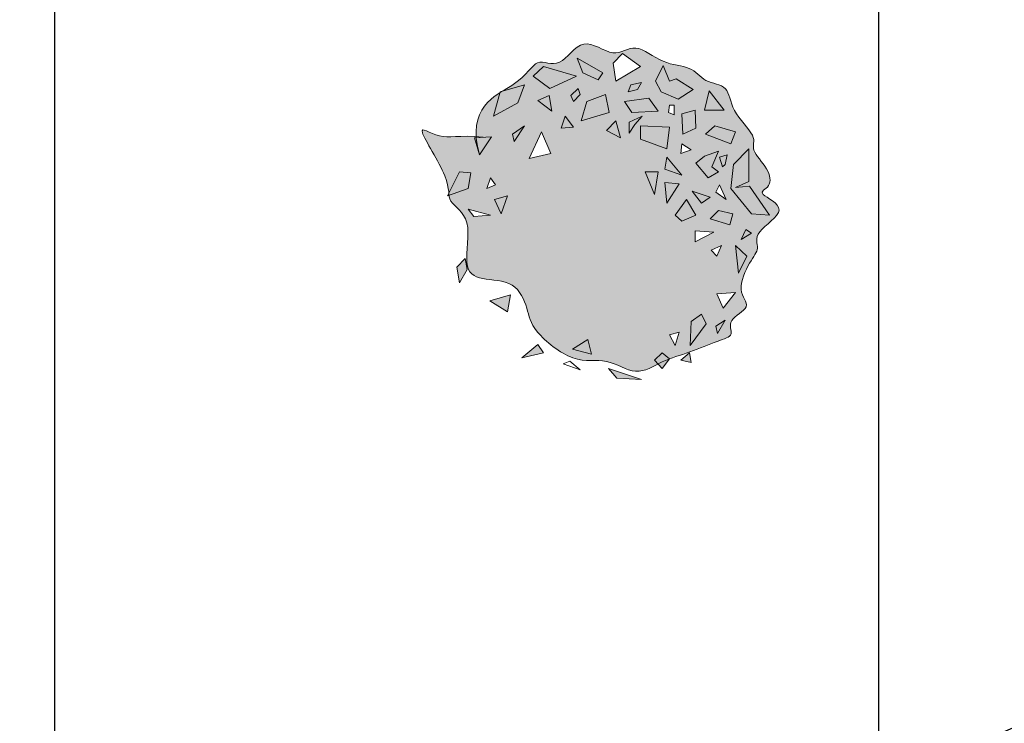
# Model space of a CAD drawing. Units: metres. Extents: x 4298.5 to 4325.2, y 2075 to 2095.8.
# Tile 4 of 35: x 4305.827 to 4307.62, y 2077.753 to 2079.034. Entities that reach past the tile are written whole.
import ezdxf

# ---------------------------------------------------------------- set-up
doc = ezdxf.new("R2010")
doc.units = ezdxf.units.M
doc.layers.add('A-ANNO-DIMS', color=2, linetype='Continuous', lineweight=18)
doc.layers.add('L-PLNT', color=94, linetype='Continuous', lineweight=13)
doc.layers.add('L-PLNT-PATT', color=116, linetype='Continuous', lineweight=13, true_color=0x13823e)
doc.styles.get("Standard").update_dxf_attribs({"font": 'arial.ttf'})
doc.dimstyles.get("Standard").update_dxf_attribs({"dimtxt": 0.18, "dimasz": 0.18, "dimexe": 0.18, "dimexo": 0.0625, "dimgap": 0.09, "dimtad": 0, "dimtih": 1, "dimtoh": 1, "dimdec": 4, "dimzin": 0, "dimdsep": 46, "dimtxsty": 'Standard', "dimcen": 0.09, "dimadec": 0, "dimazin": 0, "dimtfac": 1, "dimtdec": 4, "dimtofl": 0, "dimtmove": 0, "dimatfit": 3, "dimfxl": 1, "dimtolj": 1, "dimtzin": 0, "dimarcsym": 0})

# ---------------------------------------------------------------- blocks, each defined once
blk = doc.blocks.new('*U9')
for points in [[(1.237, 12.003), (0.562, 11.31), (0.764, 10.013), (2.519, 11.051)], [(-2.003, 11.656), (-1.598, 10.618), (-0.518, 10.099), (-0.181, 10.618), (-0.788, 10.964)], [(-4.432, 11.051), (-5.175, 10.359), (-3.96, 9.493), (-2.07, 10.359)], [(4.139, 11.137), (3.599, 10.013), (4.004, 9.234), (5.218, 8.715), (6.298, 9.407), (5.083, 10.186), (4.611, 10.013)], [(2.586, 9.926), (1.844, 9.753), (1.642, 9.234), (2.316, 9.407)], [(-5.782, 9.753), (-7.537, 9.234), (-8.009, 7.504), (-6.255, 8.455)], [(-1.935, 9.493), (-2.475, 8.974), (-2.273, 8.542), (-1.8, 9.061)], [(7.446, 9.32), (7.108, 7.936), (8.525, 7.936)], [(-4.837, 8.628), (-3.825, 7.85), (-4.027, 8.974)], [(0.022, 9.061), (-1.328, 8.542), (-1.733, 7.157), (0.292, 7.763)], [(1.372, 8.542), (3.126, 8.801), (3.801, 7.85), (1.912, 7.763)], [(4.611, 8.282), (4.544, 7.763), (4.949, 7.59), (4.949, 8.282)], [(6.433, 7.936), (5.488, 7.676), (5.556, 6.206), (6.501, 6.638)], [(-2.88, 7.504), (-3.15, 6.638), (-2.273, 6.725)], [(0.764, 7.157), (0.089, 6.465), (1.102, 5.946)], [(1.709, 6.292), (1.709, 7.071), (2.654, 7.504), (2.114, 6.898)], [(-5.782, 6.811), (-6.659, 6.206), (-6.524, 5.687)], [(-4.567, 6.379), (-5.445, 4.475), (-3.892, 4.821)], [(2.519, 6.811), (2.519, 5.86), (4.409, 5.167), (4.611, 6.725)], [(7.851, 6.811), (7.176, 6.206), (8.998, 5.514), (9.335, 6.379)], [(-8.144, 6.033), (-9.359, 5.946), (-9.022, 4.735)], [(5.488, 5.514), (5.421, 4.821), (6.163, 5.081)], [(8.12, 4.994), (7.108, 4.648), (6.501, 4.129), (7.378, 3.091), (8.12, 3.524), (7.648, 3.87)], [(10.28, 5.167), (9.2, 4.043), (8.998, 2.312), (10.482, 0.495), (11.765, 0.409), (10.348, 2.485), (9.335, 2.399), (10.28, 2.831)], [(4.409, 4.562), (4.274, 3.697), (5.488, 3.264)], [(8.728, 4.735), (8.188, 4.562), (8.39, 3.87), (8.593, 4.043)], [(-11.316, 1.793), (-9.831, 2.312), (-9.629, 3.437), (-10.439, 3.524)], [(-8.212, 3.091), (-8.482, 2.312), (-7.874, 2.572)], [(3.531, 1.88), (2.856, 3.524), (3.801, 3.524)], [(4.274, 2.745), (5.286, 2.658), (4.409, 1.274)], [(7.513, 1.707), (6.906, 1.274), (6.231, 2.139)], [(8.188, 2.572), (7.918, 2.053), (8.66, 1.534)], [(-6.997, 1.793), (-7.942, 1.534), (-7.469, 0.495)], [(5.826, 1.534), (5.016, 0.409), (5.488, -0.024), (6.501, 0.409)], [(-8.212, 0.409), (-9.426, 0.322), (-9.831, 0.841)], [(8.12, 0.755), (7.513, 0.149), (8.93, -0.283), (9.133, 0.495)], [(10.078, -0.629), (9.74, -1.322), (10.482, -0.889)], [(7.783, -0.803), (6.433, -1.495), (6.433, -0.716)], [(8.323, -1.754), (7.985, -2.533), (7.581, -2.1)], [(9.335, -1.754), (9.538, -3.744), (10.145, -2.533)], [(-10.034, -2.706), (-10.641, -3.312), (-10.439, -4.436), (-9.899, -3.485)], [(-8.279, -5.734), (-6.794, -5.302), (-6.997, -6.513)], [(9.335, -5.129), (8.458, -6.253), (7.985, -5.215)], [(6.096, -8.935), (6.163, -7.205), (6.906, -6.686), (7.243, -7.378)], [(8.053, -8.07), (8.593, -7.118), (7.918, -7.551)], [(5.286, -7.984), (4.611, -8.157), (5.016, -8.935)], [(-4.837, -8.849), (-4.432, -9.454), (-5.985, -9.801)], [(-2.34, -9.195), (-1.26, -8.503), (-0.99, -9.541)], [(4.071, -9.454), (3.531, -9.974), (4.071, -10.579), (4.611, -9.887)], [(6.028, -9.454), (5.421, -9.974), (6.163, -10.147)], [(-2.543, -10.06), (-3.015, -10.233), (-1.8, -10.666)], [(0.224, -10.579), (0.832, -11.272), (2.586, -11.358)]]:
    blk.add_lwpolyline(points, close=True)
blk = doc.blocks.new('*D47')
at = {"layer": 'A-ANNO-DIMS', "color": 0, "lineweight": -2, "transparency": 16777216}
for p, q in [((4300.4306, 2084.4956), (4300.4306, 2074.9896)), ((4322.8106, 2084.4956), (4322.8106, 2074.9896)), ((4300.6106, 2075.1696), (4311.2252, 2075.1696)), ((4322.6306, 2075.1696), (4312.016, 2075.1696))]:
    blk.add_line(p, q, dxfattribs=at)
at = {"layer": 'A-ANNO-DIMS', "color": 0, "transparency": 16777216}
for points in [[(4300.6106, 2075.1996), (4300.6106, 2075.1396), (4300.4306, 2075.1696)], [(4322.6306, 2075.1996), (4322.6306, 2075.1396), (4322.8106, 2075.1696)]]:
    blk.add_solid(points, dxfattribs=at)
at = {"layer": 'Defpoints', "color": 0, "transparency": 16777216}
for p in [(4300.4306, 2084.5581), (4322.8106, 2084.5581), (4322.8106, 2075.1696)]:
    blk.add_point(p, dxfattribs=at)
at = {"layer": 'A-ANNO-DIMS', "color": 0, "transparency": 16777216, "insert": (4311.6206, 2075.1696), "char_height": 0.18, "attachment_point": 5}
blk.add_mtext('\\A1;22.38', dxfattribs=at)
blk = doc.blocks.new('*D54')
at = {"layer": 'A-ANNO-DIMS', "color": 0, "lineweight": -2, "transparency": 16777216}
for p, q in [((4305.5981, 2079.8281), (4299.0921, 2079.8281)), ((4299.2721, 2079.6481), (4299.2721, 2078.26)), ((4299.2721, 2076.5081), (4299.2721, 2077.8961)), ((4309.0981, 2076.3281), (4299.0921, 2076.3281))]:
    blk.add_line(p, q, dxfattribs=at)
at = {"layer": 'A-ANNO-DIMS', "color": 0, "transparency": 16777216}
for points in [[(4299.2421, 2079.6481), (4299.3021, 2079.6481), (4299.2721, 2079.8281)], [(4299.2421, 2076.5081), (4299.3021, 2076.5081), (4299.2721, 2076.3281)]]:
    blk.add_solid(points, dxfattribs=at)
at = {"layer": 'Defpoints', "color": 0, "transparency": 16777216}
for p in [(4305.6606, 2079.8281), (4299.2721, 2076.3281), (4309.1606, 2076.3281)]:
    blk.add_point(p, dxfattribs=at)
at = {"layer": 'A-ANNO-DIMS', "color": 0, "transparency": 16777216, "insert": (4299.2721, 2078.0781), "char_height": 0.18, "attachment_point": 5}
blk.add_mtext('\\A1;3.5', dxfattribs=at)
blk = doc.blocks.new('*D59')
at = {"layer": 'A-ANNO-DIMS', "color": 0, "lineweight": -2, "transparency": 16777216}
for p, q in [((4305.8906, 2079.9956), (4305.8906, 2074.9896)), ((4307.3906, 2079.9956), (4307.3906, 2074.9896)), ((4306.0706, 2075.1696), (4306.3945, 2075.1696)), ((4307.2106, 2075.1696), (4306.8866, 2075.1696))]:
    blk.add_line(p, q, dxfattribs=at)
at = {"layer": 'A-ANNO-DIMS', "color": 0, "transparency": 16777216}
for points in [[(4306.0706, 2075.1996), (4306.0706, 2075.1396), (4305.8906, 2075.1696)], [(4307.2106, 2075.1996), (4307.2106, 2075.1396), (4307.3906, 2075.1696)]]:
    blk.add_solid(points, dxfattribs=at)
at = {"layer": 'Defpoints', "color": 0, "transparency": 16777216}
for p in [(4305.8906, 2080.0581), (4307.3906, 2080.0581), (4307.3906, 2075.1696)]:
    blk.add_point(p, dxfattribs=at)
at = {"layer": 'A-ANNO-DIMS', "color": 0, "transparency": 16777216, "insert": (4306.6406, 2075.1696), "char_height": 0.18, "attachment_point": 5}
blk.add_mtext('\\A1;1.5', dxfattribs=at)
blk = doc.blocks.new('*D78')
at = {"layer": 'A-ANNO-DIMS', "color": 0, "lineweight": -2, "transparency": 16777216}
for p, q in [((4312.4969, 2079.7393), (4312.4969, 2079.9193)), ((4312.4069, 2079.8293), (4312.5869, 2079.8293)), ((4305.3847, 2076.7806), (4307.8863, 2077.853)), ((4305.2047, 2076.7806), (4305.3847, 2076.7806))]:
    blk.add_line(p, q, dxfattribs=at)
at = {"layer": 'A-ANNO-DIMS', "color": 0, "transparency": 16777216}
blk.add_solid([(4307.8745, 2077.8806), (4307.8981, 2077.8254), (4308.0518, 2077.9239)], dxfattribs=at)
at = {"layer": 'Defpoints', "color": 0, "transparency": 16777216}
for p in [(4312.4969, 2079.8293), (4308.0518, 2077.9239)]:
    blk.add_point(p, dxfattribs=at)
at = {"layer": 'A-ANNO-DIMS', "color": 0, "transparency": 16777216, "insert": (4304.53, 2076.7806), "char_height": 0.18, "attachment_point": 5}
blk.add_mtext('\\A1;2X R4.836', dxfattribs=at)

msp = doc.modelspace()

# ---------------------------------------------------------------- hatches: boundary and pattern name
at = {"layer": 'L-PLNT-PATT'}
h = msp.add_hatch(color=256, dxfattribs=at)
h.dxf.hatch_style = 1
edge = h.paths.add_edge_path()
edge.add_spline(control_points=[(4306.9894, 2078.4071), (4306.992, 2078.4084), (4307.0106, 2078.4177), (4307.0464, 2078.4275), (4307.1009, 2078.4508), (4307.1303, 2078.4584), (4307.1115, 2078.4868), (4307.1641, 2078.511), (4307.1304, 2078.5374), (4307.1574, 2078.5971), (4307.1761, 2078.6166), (4307.1595, 2078.6451), (4307.2337, 2078.6899), (4307.1638, 2078.7195), (4307.1965, 2078.7271), (4307.1925, 2078.7623), (4307.1544, 2078.7989), (4307.173, 2078.8182), (4307.1199, 2078.8692), (4307.1199, 2078.9153), (4307.0721, 2078.9186), (4307.0516, 2078.9505), (4306.9984, 2078.9505), (4306.9461, 2078.9959), (4306.9113, 2078.9588), (4306.8506, 2079.0096), (4306.8107, 2078.9395), (4306.7661, 2078.9695), (4306.7518, 2078.9301), (4306.7115, 2078.9071), (4306.7051, 2078.9032)], knot_values=[0.818571, 0.818571, 0.818571, 0.818571, 0.97924, 1.97924, 2.97924, 3.97924, 4.97924, 5.97924, 6.97924, 7.97924, 8.97924, 9.97924, 10.97924, 11.97924, 12.97924, 13.97924, 14.97924, 15.97924, 16.97924, 17.97924, 18.97924, 19.97924, 20.97924, 21.97924, 22.97924, 23.97924, 24.97924, 25.97924, 26.97924, 27.16067, 27.16067, 27.16067, 27.16067], degree=3, periodic=0)
edge.add_line((4306.7051, 2078.9032), (4306.7464, 2078.9154))
edge.add_line((4306.7464, 2078.9154), (4306.7344, 2078.8824))
edge.add_line((4306.7344, 2078.8824), (4306.6898, 2078.8582))
edge.add_line((4306.6898, 2078.8582), (4306.7015, 2078.9008))
edge.add_spline(control_points=[(4306.7015, 2078.9008), (4306.6788, 2078.8862), (4306.6555, 2078.8652), (4306.6583, 2078.8208)], knot_values=[0.141368, 0.141368, 0.141368, 0.141368, 0.783694, 0.783694, 0.783694, 0.783694], degree=3, periodic=0)
edge.add_spline(control_points=[(4306.6583, 2078.8208), (4306.6622, 2078.8206), (4306.6665, 2078.8202), (4306.671, 2078.8198)], knot_values=[40.901028, 40.901028, 40.901028, 40.901028, 41, 41, 41, 41], degree=3, periodic=0)
edge.add_line((4306.671, 2078.8198), (4306.6864, 2078.8209))
edge.add_line((4306.6864, 2078.8209), (4306.6641, 2078.7879))
edge.add_line((4306.6641, 2078.7879), (4306.6556, 2078.8187))
edge.add_line((4306.6556, 2078.8187), (4306.6584, 2078.8189))
edge.add_spline(control_points=[(4306.6584, 2078.8189), (4306.6583, 2078.8195), (4306.6583, 2078.8202), (4306.6583, 2078.8208)], knot_values=[0.13204, 0.13204, 0.13204, 0.13204, 0.141368, 0.141368, 0.141368, 0.141368], degree=3, periodic=0)
edge.add_spline(control_points=[(4306.6583, 2078.8208), (4306.622, 2078.8232), (4306.5904, 2078.8133), (4306.5384, 2078.8553), (4306.6055, 2078.7528), (4306.6078, 2078.7259), (4306.6085, 2078.7184)], knot_values=[37.439141, 37.439141, 37.439141, 37.439141, 38.340169, 39.340169, 40.340169, 40.901028, 40.901028, 40.901028, 40.901028], degree=3, periodic=0)
edge.add_line((4306.6085, 2078.7184), (4306.6281, 2078.7572))
edge.add_line((4306.6281, 2078.7572), (4306.6487, 2078.7549))
edge.add_line((4306.6487, 2078.7549), (4306.6436, 2078.7264))
edge.add_line((4306.6436, 2078.7264), (4306.6089, 2078.7143))
edge.add_spline(control_points=[(4306.6089, 2078.7143), (4306.6094, 2078.7103), (4306.6125, 2078.6968), (4306.6539, 2078.6758), (4306.6324, 2078.5785), (4306.6646, 2078.5597), (4306.7309, 2078.5597), (4306.7536, 2078.5059), (4306.7571, 2078.4705), (4306.8381, 2078.4044), (4306.8964, 2078.4212), (4306.9468, 2078.3843), (4306.9759, 2078.4003), (4306.9894, 2078.4071)], knot_values=[27.16067, 27.16067, 27.16067, 27.16067, 27.490087, 28.490087, 29.490087, 30.490087, 31.490087, 32.490087, 33.490087, 34.490087, 35.490087, 36.490087, 37.329418, 37.329418, 37.329418, 37.329418], degree=3, periodic=0)
edge.add_line((4306.9894, 2078.4071), (4306.983, 2078.4143))
edge.add_line((4306.983, 2078.4143), (4306.9967, 2078.4275))
edge.add_line((4306.9967, 2078.4275), (4307.0104, 2078.4165))
h.paths.add_polyline_path([(4306.9658, 2078.7572), (4306.9898, 2078.7572), (4306.983, 2078.7154)], flags=16)
h.paths.add_polyline_path([(4307.0018, 2078.7374), (4307.0275, 2078.7352), (4307.0053, 2078.7)], flags=16)
h.paths.add_polyline_path([(4306.7944, 2078.7901), (4306.755, 2078.7813), (4306.7773, 2078.8297)], flags=16)
h.paths.add_polyline_path([(4306.9213, 2078.8187), (4306.8955, 2078.8319), (4306.9127, 2078.8494)], flags=16)
h.paths.add_polyline_path([(4307.0018, 2078.7615), (4307.0053, 2078.7835), (4307.0327, 2078.7505)], flags=16)
h.paths.add_polyline_path([(4307.0207, 2078.678), (4307.0413, 2078.7066), (4307.0584, 2078.678), (4307.0327, 2078.667)], flags=16)
h.paths.add_polyline_path([(4306.9573, 2078.8165), (4306.9573, 2078.8406), (4307.0104, 2078.8385), (4307.0053, 2078.7989)], flags=16)
h.paths.add_polyline_path([(4306.9367, 2078.8275), (4306.9367, 2078.8472), (4306.9607, 2078.8582), (4306.947, 2078.8428)], flags=16)
h.paths.add_polyline_path([(4306.8355, 2078.8385), (4306.8133, 2078.8362), (4306.8201, 2078.8582)], flags=16)
h.paths.add_polyline_path([(4306.8493, 2078.8494), (4306.8595, 2078.8846), (4306.8938, 2078.8978), (4306.9007, 2078.8648)], flags=16)
h.paths.add_polyline_path([(4306.7156, 2078.7132), (4306.7036, 2078.6802), (4306.6915, 2078.7066)], flags=16)
h.paths.add_polyline_path([(4307.0515, 2078.722), (4307.0841, 2078.711), (4307.0687, 2078.7)], flags=16)
h.paths.add_polyline_path([(4307.031, 2078.7901), (4307.0327, 2078.8077), (4307.0498, 2078.7967)], flags=16)
h.paths.add_polyline_path([(4306.9418, 2078.8648), (4306.9281, 2078.8846), (4306.9727, 2078.8912), (4306.9898, 2078.867)], flags=16)
h.paths.add_polyline_path([(4307.0567, 2078.6495), (4307.091, 2078.6472), (4307.0567, 2078.6297)], flags=16)
h.paths.add_polyline_path([(4306.6933, 2078.733), (4306.6778, 2078.7264), (4306.6847, 2078.7462)], flags=16)
h.paths.add_polyline_path([(4306.7961, 2078.867), (4306.7704, 2078.8868), (4306.791, 2078.8956)], flags=16)
h.paths.add_polyline_path([(4306.7276, 2078.8121), (4306.7241, 2078.8253), (4306.7464, 2078.8406)], flags=16)
h.paths.add_polyline_path([(4306.8355, 2078.8846), (4306.8304, 2078.8956), (4306.8441, 2078.9088), (4306.8476, 2078.8978)], flags=16)
h.paths.add_polyline_path([(4307.0584, 2078.7725), (4307.0738, 2078.7857), (4307.0995, 2078.7945), (4307.0875, 2078.7659), (4307.0995, 2078.7572), (4307.0807, 2078.7462)], flags=16)
h.paths.add_polyline_path([(4306.6847, 2078.678), (4306.6539, 2078.6758), (4306.6436, 2078.689)], flags=16)
h.paths.add_polyline_path([(4307.0344, 2078.8253), (4307.0327, 2078.8626), (4307.0567, 2078.8692), (4307.0584, 2078.8362)], flags=16)
h.paths.add_polyline_path([(4307.0841, 2078.6714), (4307.0995, 2078.6868), (4307.1253, 2078.6802), (4307.1201, 2078.6605)], flags=16)
h.paths.add_polyline_path([(4307.0087, 2078.8648), (4307.0104, 2078.878), (4307.019, 2078.878), (4307.019, 2078.8604)], flags=16)
h.paths.add_polyline_path([(4306.935, 2078.9022), (4306.9401, 2078.9154), (4306.959, 2078.9198), (4306.9521, 2078.9066)], flags=16)
h.paths.add_polyline_path([(4307.0944, 2078.7198), (4307.1012, 2078.733), (4307.1132, 2078.7066)], flags=16)
h.paths.add_polyline_path([(4307.0858, 2078.6143), (4307.1047, 2078.6231), (4307.0961, 2078.6033)], flags=16)
h.paths.add_polyline_path([(4306.8801, 2078.9242), (4306.8527, 2078.9373), (4306.8424, 2078.9637), (4306.8733, 2078.9461), (4306.8887, 2078.9373)], flags=16)
h.paths.add_polyline_path([(4306.9127, 2078.922), (4306.9075, 2078.9549), (4306.9247, 2078.9725), (4306.9573, 2078.9483)], flags=16)
h.paths.add_polyline_path([(4306.7927, 2078.9088), (4306.7618, 2078.9308), (4306.7807, 2078.9483), (4306.8407, 2078.9308)], flags=16)
h.paths.add_polyline_path([(4307.0755, 2078.8253), (4307.0927, 2078.8406), (4307.1304, 2078.8297), (4307.1218, 2078.8077)], flags=16)
h.paths.add_polyline_path([(4306.995, 2078.9022), (4306.9847, 2078.922), (4306.9984, 2078.9505), (4307.0104, 2078.922), (4307.0224, 2078.9264), (4307.0532, 2078.9066), (4307.0258, 2078.889)], flags=16)
h.paths.add_polyline_path([(4307.1064, 2078.7659), (4307.1012, 2078.7835), (4307.115, 2078.7879), (4307.1115, 2078.7703)], flags=16)
h.paths.add_polyline_path([(4307.1218, 2078.7264), (4307.127, 2078.7703), (4307.1544, 2078.7989), (4307.1544, 2078.7395), (4307.1304, 2078.7286), (4307.1561, 2078.7308), (4307.1921, 2078.678), (4307.1595, 2078.6802)], flags=16)
h.paths.add_polyline_path([(4306.8613, 2078.4517), (4306.8681, 2078.4253), (4306.8338, 2078.4341)], flags=16)
h.paths.add_polyline_path([(4307.0738, 2078.8692), (4307.0824, 2078.9044), (4307.1098, 2078.8692)], flags=16)
h.paths.add_polyline_path([(4307.1304, 2078.6231), (4307.151, 2078.6033), (4307.1355, 2078.5725)], flags=16)
h.paths.add_polyline_path([(4307.1407, 2078.6341), (4307.1493, 2078.6517), (4307.1595, 2078.6451)], flags=16)
h.paths.add_polyline_path([(4307.0104, 2078.4605), (4307.0275, 2078.4648), (4307.0207, 2078.4407)], flags=16)
h.paths.add_polyline_path([(4307.0961, 2078.5352), (4307.1304, 2078.5374), (4307.1081, 2078.5088)], flags=16)
h.paths.add_polyline_path([(4307.0498, 2078.4846), (4307.0687, 2078.4978), (4307.0772, 2078.4802), (4307.0481, 2078.4407)], flags=16)
h.paths.add_polyline_path([(4307.0944, 2078.4758), (4307.1115, 2078.4868), (4307.0978, 2078.4627)], flags=16)
h = msp.add_hatch(color=256, dxfattribs=at)
h.dxf.hatch_style = 1
h.paths.add_polyline_path([(4307.0053, 2078.7989), (4307.0104, 2078.8385), (4306.9573, 2078.8406), (4306.9573, 2078.8165)])
h.paths.add_polyline_path([(4307.0515, 2078.722), (4307.0687, 2078.7), (4307.0841, 2078.711)])
h.paths.add_polyline_path([(4307.0327, 2078.8626), (4307.0344, 2078.8253), (4307.0584, 2078.8362), (4307.0567, 2078.8692)])
h.paths.add_polyline_path([(4307.0532, 2078.9066), (4307.0224, 2078.9264), (4307.0104, 2078.922), (4306.9984, 2078.9505), (4306.9847, 2078.922), (4306.995, 2078.9022), (4307.0258, 2078.889)])
h.paths.add_polyline_path([(4306.899, 2078.3989), (4306.9144, 2078.3813), (4306.959, 2078.3791)])
h.paths.add_polyline_path([(4306.8801, 2078.9242), (4306.8887, 2078.9373), (4306.8733, 2078.9461), (4306.8424, 2078.9637), (4306.8527, 2078.9373)])
h.paths.add_polyline_path([(4306.7807, 2078.9483), (4306.7618, 2078.9308), (4306.7927, 2078.9088), (4306.8407, 2078.9308)])
h.paths.add_polyline_path([(4306.8595, 2078.8846), (4306.8493, 2078.8494), (4306.9007, 2078.8648), (4306.8938, 2078.8978)])
h.paths.add_polyline_path([(4306.8476, 2078.8978), (4306.8441, 2078.9088), (4306.8304, 2078.8956), (4306.8355, 2078.8846)])
h.paths.add_polyline_path([(4306.8201, 2078.8582), (4306.8133, 2078.8362), (4306.8355, 2078.8385)])
h.paths.add_polyline_path([(4306.7961, 2078.867), (4306.791, 2078.8956), (4306.7704, 2078.8868)])
h.paths.add_polyline_path([(4306.7018, 2078.9022), (4306.6898, 2078.8582), (4306.7344, 2078.8824), (4306.7464, 2078.9154)])
h.paths.add_polyline_path([(4306.7464, 2078.8406), (4306.7241, 2078.8253), (4306.7276, 2078.8121)])
h.paths.add_polyline_path([(4306.6556, 2078.8187), (4306.6641, 2078.7879), (4306.6864, 2078.8209)])
h.paths.add_polyline_path([(4306.6058, 2078.7132), (4306.6436, 2078.7264), (4306.6487, 2078.7549), (4306.6281, 2078.7572)])
h.paths.add_polyline_path([(4306.7156, 2078.7132), (4306.6915, 2078.7066), (4306.7036, 2078.6802)])
h.paths.add_polyline_path([(4306.6418, 2078.5791), (4306.6384, 2078.5989), (4306.623, 2078.5835), (4306.6281, 2078.555)])
h.paths.add_polyline_path([(4306.7207, 2078.533), (4306.683, 2078.522), (4306.7156, 2078.5022)])
h.paths.add_polyline_path([(4306.7413, 2078.4187), (4306.7807, 2078.4275), (4306.7704, 2078.4429)])
h.paths.add_polyline_path([(4306.8613, 2078.4517), (4306.8338, 2078.4341), (4306.8681, 2078.4253)])
h.paths.add_polyline_path([(4306.9967, 2078.4275), (4306.983, 2078.4143), (4306.9967, 2078.3989), (4307.0104, 2078.4165)])
h.paths.add_polyline_path([(4307.0772, 2078.4802), (4307.0687, 2078.4978), (4307.0498, 2078.4846), (4307.0481, 2078.4407)])
h.paths.add_polyline_path([(4307.0464, 2078.4275), (4307.031, 2078.4143), (4307.0498, 2078.4099)])
h.paths.add_polyline_path([(4307.0944, 2078.4758), (4307.0978, 2078.4627), (4307.1115, 2078.4868)])
h.paths.add_polyline_path([(4307.1355, 2078.5725), (4307.151, 2078.6033), (4307.1304, 2078.6231)])
h.paths.add_polyline_path([(4307.0207, 2078.678), (4307.0327, 2078.667), (4307.0584, 2078.678), (4307.0413, 2078.7066)])
h.paths.add_polyline_path([(4307.1595, 2078.6802), (4307.1921, 2078.678), (4307.1561, 2078.7308), (4307.1304, 2078.7286), (4307.1544, 2078.7395), (4307.1544, 2078.7989), (4307.127, 2078.7703), (4307.1218, 2078.7264)])
h.paths.add_polyline_path([(4307.0995, 2078.6868), (4307.0841, 2078.6714), (4307.1201, 2078.6605), (4307.1253, 2078.6802)])
h.paths.add_polyline_path([(4307.1595, 2078.6451), (4307.1493, 2078.6517), (4307.1407, 2078.6341)])
h.paths.add_polyline_path([(4307.0995, 2078.7945), (4307.0738, 2078.7857), (4307.0584, 2078.7725), (4307.0807, 2078.7462), (4307.0995, 2078.7572), (4307.0875, 2078.7659)])
h.paths.add_polyline_path([(4307.1012, 2078.7835), (4307.1064, 2078.7659), (4307.1115, 2078.7703), (4307.115, 2078.7879)])
h.paths.add_polyline_path([(4307.1218, 2078.8077), (4307.1304, 2078.8297), (4307.0927, 2078.8406), (4307.0755, 2078.8253)])
h.paths.add_polyline_path([(4307.0327, 2078.7505), (4307.0053, 2078.7835), (4307.0018, 2078.7615)])
h.paths.add_polyline_path([(4306.9898, 2078.7572), (4306.9658, 2078.7572), (4306.983, 2078.7154)])
h.paths.add_polyline_path([(4307.0275, 2078.7352), (4307.0018, 2078.7374), (4307.0053, 2078.7)])
h.paths.add_polyline_path([(4306.9898, 2078.867), (4306.9727, 2078.8912), (4306.9281, 2078.8846), (4306.9418, 2078.8648)])
h.paths.add_polyline_path([(4306.947, 2078.8428), (4306.9607, 2078.8582), (4306.9367, 2078.8472), (4306.9367, 2078.8275)])
h.paths.add_polyline_path([(4306.9127, 2078.8494), (4306.8955, 2078.8319), (4306.9213, 2078.8187)])
h.paths.add_polyline_path([(4306.9521, 2078.9066), (4306.959, 2078.9198), (4306.9401, 2078.9154), (4306.935, 2078.9022)])
h.paths.add_polyline_path([(4307.0824, 2078.9044), (4307.0738, 2078.8692), (4307.1098, 2078.8692)])

# ---------------------------------------------------------------- linework, layer by layer
at = {"layer": 'L-PLNT'}
msp.add_open_spline([(4306.6641, 2078.7879), (4306.64, 2078.8744), (4306.7464, 2078.9154), (4306.7661, 2078.9695), (4306.8107, 2078.9395), (4306.8506, 2079.0096), (4306.9113, 2078.9588), (4306.9461, 2078.9959), (4306.9984, 2078.9505), (4307.0516, 2078.9505), (4307.0721, 2078.9186), (4307.1199, 2078.9153), (4307.1199, 2078.8692), (4307.173, 2078.8182), (4307.1544, 2078.7989), (4307.1925, 2078.7623), (4307.1965, 2078.7271), (4307.1638, 2078.7195), (4307.2337, 2078.6899), (4307.1595, 2078.6451), (4307.1761, 2078.6166), (4307.1574, 2078.5971), (4307.1304, 2078.5374), (4307.1641, 2078.511), (4307.1115, 2078.4868), (4307.1303, 2078.4584), (4307.1009, 2078.4508), (4307.0464, 2078.4275), (4306.9967, 2078.4139), (4306.9496, 2078.3822), (4306.8964, 2078.4212), (4306.8381, 2078.4044), (4306.7571, 2078.4705), (4306.7536, 2078.5059), (4306.7309, 2078.5597), (4306.6646, 2078.5597), (4306.6324, 2078.5785), (4306.6539, 2078.6758), (4306.6006, 2078.7028), (4306.617, 2078.7352), (4306.5384, 2078.8553), (4306.5922, 2078.8119), (4306.6253, 2078.8243), (4306.671, 2078.8198)], degree=3, dxfattribs=at)

# ---------------------------------------------------------------- block references
at = {"layer": 'L-PLNT', "xscale": 0.0254, "yscale": 0.0254, "zscale": 0.0254}
msp.add_blockref('*U9', (4306.8933, 2078.6676), dxfattribs=at)

# ---------------------------------------------------------------- dimensions: what is measured, and where the dimension line sits
at = {"layer": 'A-ANNO-DIMS'}
for base, p1, p2, override, picture, middle in [((4322.8106, 2075.1696), (4300.4306, 2084.5581), (4322.8106, 2084.5581), {"dimdec": 2, "dimlfac": 1, "dimrnd": 0, "dimzin": 0, "dimdsep": 46, "dimlunit": 2}, '*D47', (4311.6206, 2075.1696)), ((4307.3906, 2075.1696), (4305.8906, 2080.0581), (4307.3906, 2080.0581), {"dimdec": 1, "dimlfac": 1, "dimrnd": 0, "dimzin": 0, "dimdsep": 46, "dimlunit": 2}, '*D59', (4306.6406, 2075.1696))]:
    dim = msp.add_linear_dim(base=base, p1=p1, p2=p2, dimstyle='Standard', override=override, dxfattribs=at)
    dim.commit()
    dim.dimension.update_dxf_attribs({"geometry": picture, "text_midpoint": middle})
dim = msp.add_radius_dim(center=(4312.4969, 2079.8293), mpoint=(4308.0518, 2077.9239), text='2X <>', dimstyle='Standard', override={"dimdec": 3, "dimlfac": 1, "dimrnd": 0, "dimzin": 0, "dimdsep": 46, "dimlunit": 2}, dxfattribs=at)
dim.commit()
dim.dimension.update_dxf_attribs({"geometry": '*D78', "text_midpoint": (4304.53, 2076.7806), "dimtype": 164})
dim = msp.add_linear_dim(base=(4299.2721, 2076.3281), p1=(4305.6606, 2079.8281), p2=(4309.1606, 2076.3281), angle=90, dimstyle='Standard', override={"dimdec": 1, "dimlfac": 1, "dimrnd": 0, "dimzin": 0, "dimdsep": 46, "dimlunit": 2}, dxfattribs=at)
dim.commit()
dim.dimension.update_dxf_attribs({"geometry": '*D54', "text_midpoint": (4299.2721, 2078.0781)})

doc.saveas('drawing.dxf')
